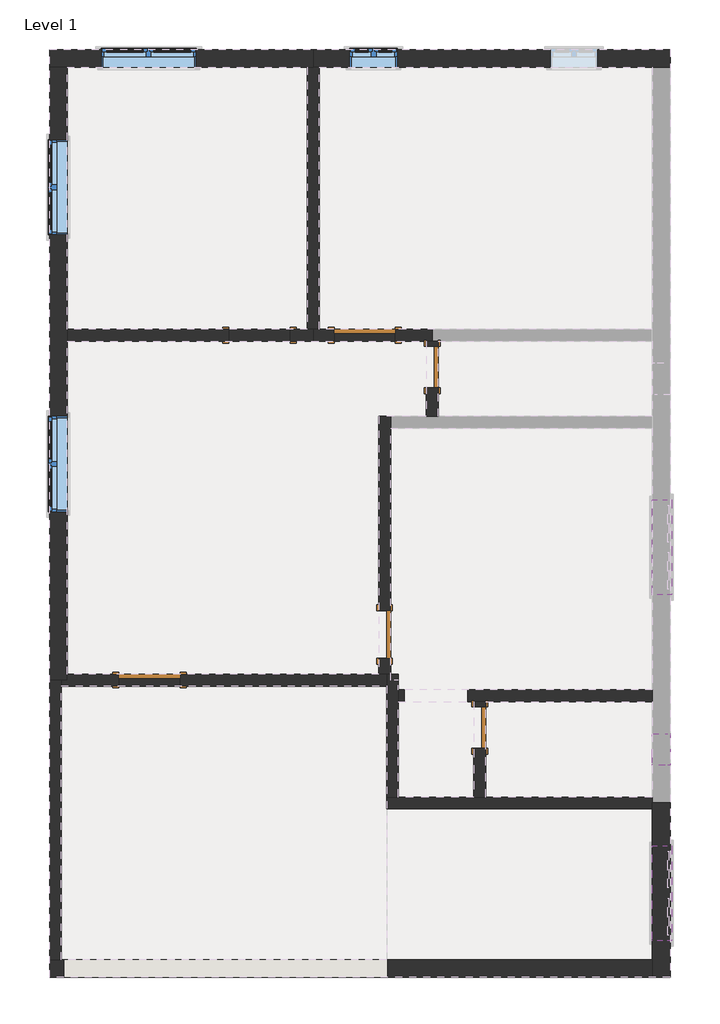
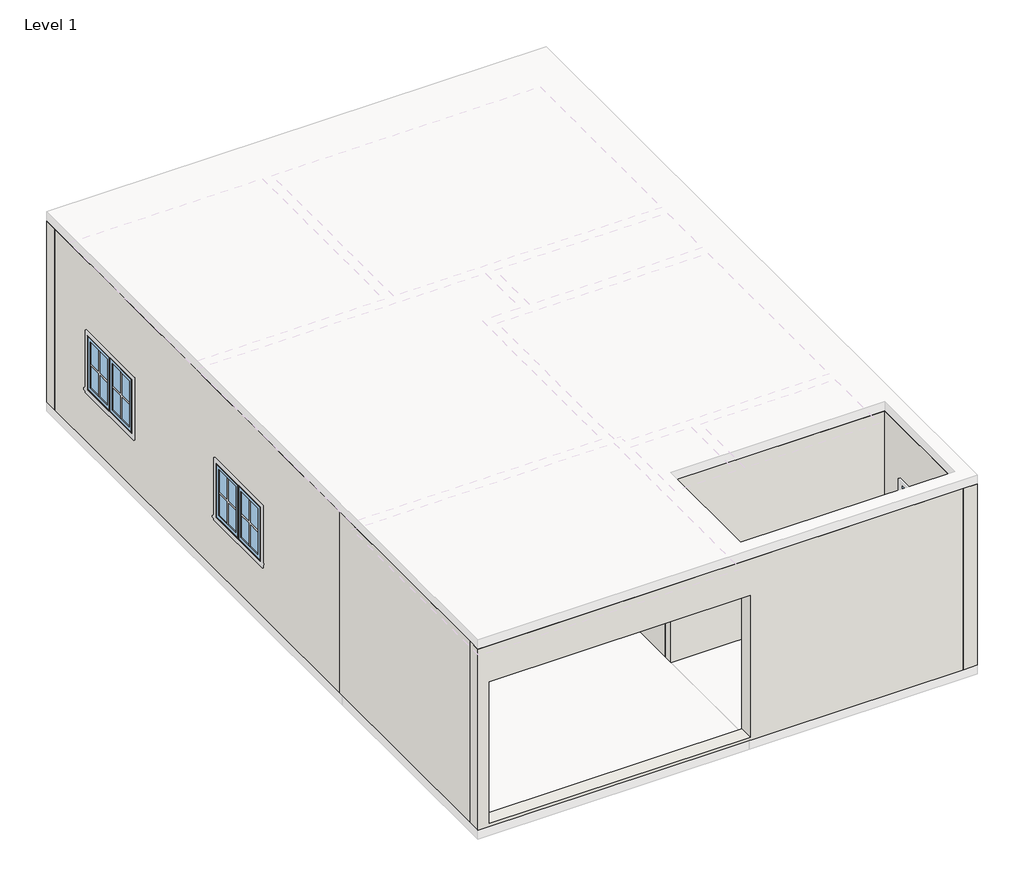
# One storey, part 1 of 2: 24 walls, 10 windows, 6 doors.
"""IFC4 building model written with IfcOpenShell, lengths in millimetres."""

from ifc_helpers import new_model, si_unit, frame, origin, origin_with_axes, place, context, project, spatial, polyline, outline, extrude, faceted_brep, transform, mapped, element, save
from components import door_2908be75, door_9ea4ff49, door_dc34e247, door_b804d09e, fixed_2_415b3208, window_casement_double_3_c417fced, window_casement_double_4_c19c33cb

model = new_model("IFC4")

# Units and contexts
model_context = context("Model", 3, world=origin())
ifc_project = project(units=[si_unit("LENGTHUNIT", "METRE", prefix="MILLI")], contexts=[model_context])

# Site, building, storey
site = spatial("IfcSite", under=ifc_project)
building = spatial("IfcBuilding", under=site)
storey = spatial("IfcBuildingStorey", under=building, Name="Level 1", Elevation=0.0)

# Doors
placement = place(None, origin())
door_shape = door_2908be75(model_context)
element("IfcDoor", 1, ObjectType="Single-Flush : 1' 9\"", at=placement, inside=storey, context=model_context, shape_type="MappedRepresentation", body=[
    mapped(door_shape, transform((-397.3154463, -2781.5544725, 0.0), x_axis=(0.0, 1.0, 0.0), y_axis=(-1.0, 0.0, 0.0), z_axis=(0.0, 0.0, 1.0))),
])
element("IfcDoor", 2, ObjectType="Single-Flush : 1' 9\"", at=placement, inside=storey, context=model_context, shape_type="MappedRepresentation", body=[
    mapped(door_shape, transform((-1006.9154463, 1841.2455275, 0.0), x_axis=(0.0, 1.0, 0.0), y_axis=(-1.0, 0.0, 0.0), z_axis=(0.0, 0.0, 1.0))),
])
door_2_shape = door_9ea4ff49(model_context)
element("IfcDoor", 3, ObjectType="Single-Flush : 2'0\"", at=placement, inside=storey, context=model_context, shape_type="MappedRepresentation", body=[
    mapped(door_2_shape, transform((-1616.5154463, -1587.7544725, 0.0), x_axis=(0.0, -1.0, 0.0), y_axis=(1.0, 0.0, 0.0), z_axis=(0.0, 0.0, 1.0))),
])
door_3_shape = door_dc34e247(model_context)
element("IfcDoor", 4, ObjectType="Single-Flush : 2'7\"", at=placement, inside=storey, context=model_context, shape_type="MappedRepresentation", body=[
    mapped(door_3_shape, transform((-4626.4154463, -2171.9544725, 0.0), x_axis=(-1.0, 0.0, 0.0), y_axis=(0.0, -1.0, 0.0), z_axis=(0.0, 0.0, 1.0))),
])
element("IfcDoor", 5, ObjectType="Single-Flush : 2'7\"", at=placement, inside=storey, context=model_context, shape_type="MappedRepresentation", body=[
    mapped(door_3_shape, transform((-1870.5154463, 2247.6455275, 0.0), x_axis=(-1.0, 0.0, 0.0), y_axis=(0.0, -1.0, 0.0), z_axis=(0.0, 0.0, 1.0))),
])
door_4_shape = door_b804d09e(model_context)
element("IfcDoor", 6, ObjectType="Single-Flush : 2'7\"", at=placement, inside=storey, context=model_context, shape_type="MappedRepresentation", body=[
    mapped(door_4_shape, transform((-3216.7154463, 2247.6455275, 0.0), x_axis=(1.0, 0.0, 0.0), y_axis=(0.0, 1.0, 0.0), z_axis=(0.0, 0.0, 1.0))),
])

# Walls
element("IfcWall", 7, ObjectType="Generic - 6\"", at=placement, inside=storey, context=model_context, shape_type="Brep", body=[
    faceted_brep([(-5909.1154463, -2171.9544725, 0.0), (-5909.1154463, -5753.3544725, 0.0), (-5909.1154463, -5753.3544725, 3048.0), (-5909.1154463, -2171.9544725, 3048.0), (-5756.7154463, -2171.9544725, 0.0), (-5756.7154463, -2171.9544725, 3048.0), (-5756.7154463, -2248.1544725, 3048.0), (-5756.7154463, -5753.3544725, 3048.0), (-5756.7154463, -5753.3544725, 0.0), (-5756.7154463, -2248.1544725, 0.0)], [[[0, 1, 2, 3]], [[4, 5, 6, 7, 8, 9]], [[1, 0, 4, 9, 8]], [[3, 2, 7, 6, 5]], [[0, 3, 5, 4]], [[2, 1, 8, 7]]]),
])
element("IfcWall", 8, ObjectType="Generic - 6\"", at=placement, inside=storey, context=model_context, shape_type="Brep", body=[
    faceted_brep([(1812.4845537, -3670.5544725, 0.0), (-321.1154463, -3670.5544725, 0.0), (-473.5154463, -3670.5544725, 0.0), (-1438.7154463, -3670.5544725, 0.0), (-1591.1154463, -3670.5544725, 0.0), (-1591.1154463, -3670.5544725, 3048.0), (-1438.7154463, -3670.5544725, 3048.0), (-473.5154463, -3670.5544725, 3048.0), (-321.1154463, -3670.5544725, 3048.0), (1812.4845537, -3670.5544725, 3048.0), (1812.4845537, -3822.9544725, 0.0), (1812.4845537, -3822.9544725, 3048.0), (-1591.1154463, -3822.9544725, 3048.0), (-1591.1154463, -3822.9544725, 0.0), (1812.4845537, -3746.7544725, 0.0), (1812.4845537, -3746.7544725, 3048.0)], [[[0, 1, 2, 3, 4, 5, 6, 7, 8, 9]], [[10, 11, 12, 13]], [[4, 3, 2, 1, 0, 14, 10, 13]], [[9, 8, 7, 6, 5, 12, 11, 15]], [[5, 4, 13, 12]], [[0, 9, 15, 11, 10, 14]]]),
])
element("IfcWall", 9, ObjectType="Generic - 6\"", at=placement, inside=storey, context=model_context, shape_type="Brep", body=[
    faceted_brep([(-1438.7154463, -3670.5544725, 0.0), (-1438.7154463, -2451.3544725, 0.0), (-1438.7154463, -2298.9544725, 0.0), (-1438.7154463, -2095.7544725, 0.0), (-1438.7154463, -2095.7544725, 3048.0), (-1438.7154463, -2298.9544725, 3048.0), (-1438.7154463, -2451.3544725, 3048.0), (-1438.7154463, -3670.5544725, 3048.0), (-1591.1154463, -3670.5544725, 0.0), (-1591.1154463, -3670.5544725, 3048.0), (-1591.1154463, -2248.1544725, 3048.0), (-1591.1154463, -2171.9544725, 3048.0), (-1591.1154463, -2095.7544725, 3048.0), (-1591.1154463, -2095.7544725, 0.0), (-1591.1154463, -2171.9544725, 0.0), (-1591.1154463, -2248.1544725, 0.0), (-1540.3154463, -2095.7544725, 0.0), (-1540.3154463, -2095.7544725, 3048.0)], [[[0, 1, 2, 3, 4, 5, 6, 7]], [[8, 9, 10, 11, 12, 13, 14, 15]], [[3, 2, 1, 0, 8, 15, 14, 13, 16]], [[7, 6, 5, 4, 17, 12, 11, 10, 9]], [[0, 7, 9, 8]], [[4, 3, 16, 13, 12, 17]]]),
])
element("IfcWall", 10, ObjectType="Generic - 6\"", at=placement, inside=storey, context=model_context, shape_type="Brep", body=[
    faceted_brep([(-5020.1154463, -2095.7544725, 2133.6), (-5020.1154463, -2095.7544725, 0.0), (-5680.5154463, -2095.7544725, 0.0), (-5680.5154463, -2095.7544725, 3048.0), (-1692.7154463, -2095.7544725, 3048.0), (-1591.1154463, -2095.7544725, 3048.0), (-1591.1154463, -2095.7544725, 0.0), (-1692.7154463, -2095.7544725, 0.0), (-4232.7154463, -2095.7544725, 0.0), (-4232.7154463, -2095.7544725, 2133.6), (-5756.7154463, -2248.1544725, 0.0), (-5020.1154463, -2248.1544725, 0.0), (-5020.1154463, -2248.1544725, 2133.6), (-4232.7154463, -2248.1544725, 2133.6), (-4232.7154463, -2248.1544725, 0.0), (-1591.1154463, -2248.1544725, 0.0), (-1591.1154463, -2248.1544725, 3048.0), (-5756.7154463, -2248.1544725, 3048.0), (-5756.7154463, -2171.9544725, 0.0), (-5680.5154463, -2171.9544725, 0.0), (-5680.5154463, -2171.9544725, 3048.0), (-5756.7154463, -2171.9544725, 3048.0)], [[[0, 1, 2, 3, 4, 5, 6, 7, 8, 9]], [[10, 11, 12, 13, 14, 15, 16, 17]], [[2, 1, 11, 10, 18, 19]], [[8, 7, 6, 15, 14]], [[5, 4, 3, 20, 21, 17, 16]], [[3, 2, 19, 20]], [[19, 18, 21, 20]], [[18, 10, 17, 21]], [[6, 5, 16, 15]], [[12, 11, 1, 0]], [[13, 12, 0, 9]], [[14, 13, 9, 8]]]),
])
element("IfcWall", 11, ObjectType="Generic - 6\"", at=placement, inside=storey, context=model_context, shape_type="Brep", body=[
    faceted_brep([(1812.4845537, -2451.3544725, 0.0), (1812.4845537, -2451.3544725, 3048.0), (-321.1154463, -2451.3544725, 3048.0), (-473.5154463, -2451.3544725, 3048.0), (-1438.7154463, -2451.3544725, 3048.0), (-1438.7154463, -2451.3544725, 0.0), (-1367.0206652, -2451.3544725, 0.0), (-1367.0206652, -2451.3544725, 2438.4), (-547.4818767, -2451.3544725, 2438.4), (-547.4818767, -2451.3544725, 0.0), (-473.5154463, -2451.3544725, 0.0), (-321.1154463, -2451.3544725, 0.0), (1812.4845537, -2298.9544725, 3048.0), (1812.4845537, -2298.9544725, 0.0), (-547.4818767, -2298.9544725, 0.0), (-547.4818767, -2298.9544725, 2438.4), (-1367.0206652, -2298.9544725, 2438.4), (-1367.0206652, -2298.9544725, 0.0), (-1438.7154463, -2298.9544725, 0.0), (-1438.7154463, -2298.9544725, 3048.0)], [[[0, 1, 2, 3, 4, 5, 6, 7, 8, 9, 10, 11]], [[12, 13, 14, 15, 16, 17, 18, 19]], [[5, 18, 17, 6]], [[13, 0, 11, 10, 9, 14]], [[4, 3, 2, 1, 12, 19]], [[1, 0, 13, 12]], [[5, 4, 19, 18]], [[7, 16, 15, 8]], [[16, 7, 6, 17]], [[8, 15, 14, 9]]]),
])
element("IfcWall", 12, ObjectType="Generic - 6\"", at=placement, inside=storey, context=model_context, shape_type="SweptSolid", body=[
    extrude(outline(polyline([(-2451.3544725, 0.0), (-2514.8544725, 0.0), (-2514.8544725, 2133.6), (-3048.2544725, 2133.6), (-3048.2544725, 0.0), (-3670.5544725, 0.0), (-3670.5544725, 3048.0), (-2451.3544725, 3048.0), (-2451.3544725, 0.0)])), frame((-473.5154463, 0.0, 0.0), z_axis=(1.0, 0.0, 0.0), x_axis=(0.0, 1.0, 0.0)), (0.0, 0.0, 1.0), 152.4),
])
element("IfcWall", 13, ObjectType="Generic - 6\"", at=placement, inside=storey, context=model_context, shape_type="Brep", body=[
    faceted_brep([(-1540.3154463, -2095.7544725, 0.0), (-1540.3154463, -1892.5544725, 0.0), (-1540.3154463, -1892.5544725, 2133.6), (-1540.3154463, -1282.9544725, 2133.6), (-1540.3154463, -1282.9544725, 0.0), (-1540.3154463, 1053.8455275, 0.0), (-1540.3154463, 1206.2455275, 0.0), (-1540.3154463, 1206.2455275, 3048.0), (-1540.3154463, 1053.8455275, 3048.0), (-1540.3154463, -2095.7544725, 3048.0), (-1692.7154463, -1892.5544725, 2133.6), (-1692.7154463, -1892.5544725, 0.0), (-1692.7154463, -2095.7544725, 0.0), (-1692.7154463, -2095.7544725, 3048.0), (-1692.7154463, 1206.2455275, 3048.0), (-1692.7154463, 1206.2455275, 0.0), (-1692.7154463, -1282.9544725, 0.0), (-1692.7154463, -1282.9544725, 2133.6), (-1591.1154463, -2095.7544725, 0.0), (-1591.1154463, -2095.7544725, 3048.0)], [[[0, 1, 2, 3, 4, 5, 6, 7, 8, 9]], [[10, 11, 12, 13, 14, 15, 16, 17]], [[16, 15, 6, 5, 4]], [[12, 11, 1, 0, 18]], [[9, 8, 7, 14, 13, 19]], [[0, 9, 19, 13, 12, 18]], [[7, 6, 15, 14]], [[2, 1, 11, 10]], [[3, 2, 10, 17]], [[4, 3, 17, 16]]]),
])
element("IfcWall", 14, ObjectType="Generic - 6\"", at=placement, inside=storey, context=model_context, shape_type="Brep", body=[
    faceted_brep([(-930.7154463, 2107.9455275, 2133.6), (-930.7154463, 2107.9455275, 0.0), (-930.7154463, 2171.4455275, 0.0), (-930.7154463, 2171.4455275, 3048.0), (-930.7154463, 1206.2455275, 3048.0), (-930.7154463, 1206.2455275, 0.0), (-930.7154463, 1574.5455275, 0.0), (-930.7154463, 1574.5455275, 2133.6), (-1083.1154463, 2171.4455275, 0.0), (-1083.1154463, 2107.9455275, 0.0), (-1083.1154463, 2107.9455275, 2133.6), (-1083.1154463, 1574.5455275, 2133.6), (-1083.1154463, 1574.5455275, 0.0), (-1083.1154463, 1206.2455275, 0.0), (-1083.1154463, 1206.2455275, 3048.0), (-1083.1154463, 2171.4455275, 3048.0), (-1006.9154463, 2171.4455275, 0.0), (-1006.9154463, 2171.4455275, 3048.0)], [[[0, 1, 2, 3, 4, 5, 6, 7]], [[8, 9, 10, 11, 12, 13, 14, 15]], [[6, 5, 13, 12]], [[2, 1, 9, 8, 16]], [[4, 3, 17, 15, 14]], [[5, 4, 14, 13]], [[10, 9, 1, 0]], [[11, 10, 0, 7]], [[12, 11, 7, 6]], [[3, 2, 16, 8, 15, 17]]]),
])
element("IfcWall", 15, ObjectType="Generic - 6\"", at=placement, inside=storey, context=model_context, shape_type="Brep", body=[
    faceted_brep([(-2607.1154463, 5678.2330275, 0.0), (-2607.1154463, 2323.8455275, 0.0), (-2607.1154463, 2323.8455275, 3048.0), (-2607.1154463, 5678.2330275, 3048.0), (-2454.7154463, 5678.2330275, 0.0), (-2454.7154463, 5678.2330275, 3048.0), (-2454.7154463, 2323.8455275, 3048.0), (-2454.7154463, 2323.8455275, 0.0), (-2530.9154463, 5678.2330275, 0.0), (-2530.9154463, 2323.8455275, 0.0), (-2530.9154463, 2323.8455275, 3048.0), (-2530.9154463, 5678.2330275, 3048.0)], [[[0, 1, 2, 3]], [[4, 5, 6, 7]], [[1, 0, 8, 4, 7, 9]], [[3, 2, 10, 6, 5, 11]], [[0, 3, 11, 5, 4, 8]], [[2, 1, 9, 7, 6, 10]]]),
])
element("IfcWall", 16, ObjectType="Generic - 6\"", at=placement, inside=storey, context=model_context, shape_type="Brep", body=[
    faceted_brep([(-2530.9154463, 2323.8455275, 0.0), (-2607.1154463, 2323.8455275, 0.0), (-2823.0154463, 2323.8455275, 0.0), (-2823.0154463, 2323.8455275, 2133.6), (-3610.4154463, 2323.8455275, 2133.6), (-3610.4154463, 2323.8455275, 0.0), (-5680.5154463, 2323.8455275, 0.0), (-5680.5154463, 2323.8455275, 3048.0), (-2607.1154463, 2323.8455275, 3048.0), (-2530.9154463, 2323.8455275, 3048.0), (-2823.0154463, 2171.4455275, 2133.6), (-2823.0154463, 2171.4455275, 0.0), (-2530.9154463, 2171.4455275, 0.0), (-2530.9154463, 2171.4455275, 3048.0), (-5680.5154463, 2171.4455275, 3048.0), (-5680.5154463, 2171.4455275, 0.0), (-3610.4154463, 2171.4455275, 0.0), (-3610.4154463, 2171.4455275, 2133.6)], [[[0, 1, 2, 3, 4, 5, 6, 7, 8, 9]], [[10, 11, 12, 13, 14, 15, 16, 17]], [[16, 15, 6, 5]], [[12, 11, 2, 1, 0]], [[9, 8, 7, 14, 13]], [[0, 9, 13, 12]], [[7, 6, 15, 14]], [[5, 4, 17, 16]], [[4, 3, 10, 17]], [[3, 2, 11, 10]]]),
])
element("IfcWall", 17, ObjectType="Generic - 6\"", at=placement, inside=storey, context=model_context, shape_type="Brep", body=[
    faceted_brep([(-2264.2154463, 2323.8455275, 2133.6), (-2264.2154463, 2323.8455275, 0.0), (-2454.7154463, 2323.8455275, 0.0), (-2530.9154463, 2323.8455275, 0.0), (-2530.9154463, 2323.8455275, 3048.0), (-2454.7154463, 2323.8455275, 3048.0), (-1006.9154463, 2323.8455275, 3048.0), (-1006.9154463, 2323.8455275, 0.0), (-1476.8154463, 2323.8455275, 0.0), (-1476.8154463, 2323.8455275, 2133.6), (-2530.9154463, 2171.4455275, 0.0), (-2264.2154463, 2171.4455275, 0.0), (-2264.2154463, 2171.4455275, 2133.6), (-1476.8154463, 2171.4455275, 2133.6), (-1476.8154463, 2171.4455275, 0.0), (-1083.1154463, 2171.4455275, 0.0), (-1006.9154463, 2171.4455275, 0.0), (-1006.9154463, 2171.4455275, 3048.0), (-1083.1154463, 2171.4455275, 3048.0), (-2530.9154463, 2171.4455275, 3048.0)], [[[0, 1, 2, 3, 4, 5, 6, 7, 8, 9]], [[10, 11, 12, 13, 14, 15, 16, 17, 18, 19]], [[8, 7, 16, 15, 14]], [[3, 2, 1, 11, 10]], [[4, 3, 10, 19]], [[6, 5, 4, 19, 18, 17]], [[7, 6, 17, 16]], [[14, 13, 9, 8]], [[13, 12, 0, 9]], [[12, 11, 1, 0]]]),
])
element("IfcWall", 18, ObjectType="Generic - 6\"", at=placement, inside=storey, context=model_context, shape_type="SweptSolid", body=[
    extrude(outline(polyline([(-5680.5154463, -2095.7544725), (-1692.7154463, -2095.7544725), (-1692.7154463, -2171.9544725), (-1591.1154463, -2171.9544725), (-1591.1154463, -2248.1544725), (-5756.7154463, -2248.1544725), (-5756.7154463, -2171.9544725), (-5680.5154463, -2171.9544725), (-5680.5154463, -2095.7544725)])), origin_with_axes(), (0.0, 0.0, 1.0), 3048.0),
])
element("IfcWall", 19, ObjectType="Generic - 6\"", at=placement, inside=storey, context=model_context, shape_type="Brep", body=[
    faceted_brep([(-2607.1154463, 5678.2330275, 0.0), (-2607.1154463, 2323.8455275, 0.0), (-2607.1154463, 2323.8455275, 3048.0), (-2607.1154463, 5678.2330275, 3048.0), (-2454.7154463, 5678.2330275, 0.0), (-2454.7154463, 5678.2330275, 3048.0), (-2454.7154463, 2323.8455275, 3048.0), (-2454.7154463, 2323.8455275, 0.0), (-2530.9154463, 5678.2330275, 0.0), (-2530.9154463, 2323.8455275, 0.0), (-2530.9154463, 2323.8455275, 3048.0), (-2530.9154463, 5678.2330275, 3048.0)], [[[0, 1, 2, 3]], [[4, 5, 6, 7]], [[1, 0, 8, 4, 7, 9]], [[3, 2, 10, 6, 5, 11]], [[0, 3, 11, 5, 4, 8]], [[2, 1, 9, 7, 6, 10]]]),
])
element("IfcWall", 20, ObjectType="Generic - 6\"", at=placement, inside=storey, context=model_context, shape_type="Brep", body=[
    faceted_brep([(-2530.9154463, 2323.8455275, 0.0), (-2607.1154463, 2323.8455275, 0.0), (-5680.5154463, 2323.8455275, 0.0), (-5680.5154463, 2323.8455275, 3048.0), (-2607.1154463, 2323.8455275, 3048.0), (-2530.9154463, 2323.8455275, 3048.0), (-2530.9154463, 2171.4455275, 0.0), (-2530.9154463, 2171.4455275, 3048.0), (-5680.5154463, 2171.4455275, 3048.0), (-5680.5154463, 2171.4455275, 0.0)], [[[0, 1, 2, 3, 4, 5]], [[6, 7, 8, 9]], [[2, 1, 0, 6, 9]], [[5, 4, 3, 8, 7]], [[0, 5, 7, 6]], [[3, 2, 9, 8]]]),
])
element("IfcWall", 21, ObjectType="Generic - 6\"", at=placement, inside=storey, context=model_context, shape_type="Brep", body=[
    faceted_brep([(-1006.9154463, 2323.8455275, 0.0), (-2454.7154463, 2323.8455275, 0.0), (-2530.9154463, 2323.8455275, 0.0), (-2530.9154463, 2323.8455275, 3048.0), (-2454.7154463, 2323.8455275, 3048.0), (-1006.9154463, 2323.8455275, 3048.0), (-1006.9154463, 2171.4455275, 0.0), (-1006.9154463, 2171.4455275, 3048.0), (-1083.1154463, 2171.4455275, 3048.0), (-2530.9154463, 2171.4455275, 3048.0), (-2530.9154463, 2171.4455275, 0.0), (-1083.1154463, 2171.4455275, 0.0)], [[[0, 1, 2, 3, 4, 5]], [[6, 7, 8, 9, 10, 11]], [[2, 1, 0, 6, 11, 10]], [[3, 2, 10, 9]], [[5, 4, 3, 9, 8, 7]], [[0, 5, 7, 6]]]),
])
element("IfcWall", 22, ObjectType="Generic - 9\"", at=placement, inside=storey, context=model_context, shape_type="Brep", body=[
    faceted_brep([(-5909.1154463, 5678.2330275, 0.0), (-5680.5154463, 5678.2330275, 0.0), (-2607.1154463, 5678.2330275, 0.0), (-2530.9154463, 5678.2330275, 0.0), (-2530.9154463, 5678.2330275, 3048.0), (-2607.1154463, 5678.2330275, 3048.0), (-5680.5154463, 5678.2330275, 3048.0), (-5909.1154463, 5678.2330275, 3048.0), (-4029.5154463, 5678.2330275, 1828.8), (-4029.5154463, 5678.2330275, 914.4), (-5248.7154463, 5678.2330275, 914.4), (-5248.7154463, 5678.2330275, 1828.8), (-5909.1154463, 5906.8330275, 0.0), (-5909.1154463, 5906.8330275, 3048.0), (-2530.9154463, 5906.8330275, 3048.0), (-2530.9154463, 5906.8330275, 0.0), (-4029.5154463, 5906.8330275, 1828.8), (-5248.7154463, 5906.8330275, 1828.8), (-5248.7154463, 5906.8330275, 914.4), (-4029.5154463, 5906.8330275, 914.4)], [[[0, 1, 2, 3, 4, 5, 6, 7], [8, 9, 10, 11]], [[12, 13, 14, 15], [16, 17, 18, 19]], [[3, 2, 1, 0, 12, 15]], [[4, 3, 15, 14]], [[7, 6, 5, 4, 14, 13]], [[0, 7, 13, 12]], [[9, 8, 16, 19]], [[10, 9, 19, 18]], [[11, 10, 18, 17]], [[8, 11, 17, 16]]]),
])
element("IfcWall", 23, ObjectType="Generic - 9\"", at=placement, inside=storey, context=model_context, shape_type="Brep", body=[
    faceted_brep([(1812.4845537, -5753.3544725, 0.0), (-5756.7154463, -5753.3544725, 0.0), (-5909.1154463, -5753.3544725, 0.0), (-5909.1154463, -5753.3544725, 3048.0), (-5756.7154463, -5753.3544725, 3048.0), (1812.4845537, -5753.3544725, 3048.0), (-1576.8982041, -5753.3544725, 2438.4), (-5729.1673724, -5753.3544725, 2438.4), (-5729.1673724, -5753.3544725, 50.8), (-1576.8982041, -5753.3544725, 50.8), (-5909.1154463, -5981.9544725, 0.0), (1812.4845537, -5981.9544725, 0.0), (1812.4845537, -5981.9544725, 3048.0), (-5909.1154463, -5981.9544725, 3048.0), (-5729.1673724, -5981.9544725, 2438.4), (-1576.8982041, -5981.9544725, 2438.4), (-1576.8982041, -5981.9544725, 50.8), (-5729.1673724, -5981.9544725, 50.8)], [[[0, 1, 2, 3, 4, 5], [6, 7, 8, 9]], [[10, 11, 12, 13], [14, 15, 16, 17]], [[2, 1, 0, 11, 10]], [[5, 4, 3, 13, 12]], [[0, 5, 12, 11]], [[6, 15, 14, 7]], [[8, 17, 16, 9]], [[15, 6, 9, 16]], [[7, 14, 17, 8]], [[3, 2, 10, 13]]]),
])
element("IfcWall", 24, ObjectType="Generic - 9\"", at=placement, inside=storey, context=model_context, shape_type="Brep", body=[
    faceted_brep([(-5909.1154463, 5678.2330275, 0.0), (-5909.1154463, -2171.9544725, 0.0), (-5909.1154463, -2171.9544725, 3048.0), (-5909.1154463, 5678.2330275, 3048.0), (-5909.1154463, 4751.1330275, 1828.8), (-5909.1154463, 3531.9330275, 1828.8), (-5909.1154463, 3531.9330275, 914.4), (-5909.1154463, 4751.1330275, 914.4), (-5909.1154463, 1206.2455275, 1828.8), (-5909.1154463, -12.9544725, 1828.8), (-5909.1154463, -12.9544725, 914.4), (-5909.1154463, 1206.2455275, 914.4), (-5680.5154463, 5678.2330275, 0.0), (-5680.5154463, 5678.2330275, 3048.0), (-5680.5154463, 2323.8455275, 3048.0), (-5680.5154463, 2171.4455275, 3048.0), (-5680.5154463, -2095.7544725, 3048.0), (-5680.5154463, -2171.9544725, 3048.0), (-5680.5154463, -2171.9544725, 0.0), (-5680.5154463, -2095.7544725, 0.0), (-5680.5154463, 2171.4455275, 0.0), (-5680.5154463, 2323.8455275, 0.0), (-5680.5154463, 4751.1330275, 1828.8), (-5680.5154463, 4751.1330275, 914.4), (-5680.5154463, 3531.9330275, 914.4), (-5680.5154463, 3531.9330275, 1828.8), (-5680.5154463, 1206.2455275, 1828.8), (-5680.5154463, 1206.2455275, 914.4), (-5680.5154463, -12.9544725, 914.4), (-5680.5154463, -12.9544725, 1828.8), (-5756.7154463, -2171.9544725, 0.0), (-5756.7154463, -2171.9544725, 3048.0)], [[[0, 1, 2, 3], [4, 5, 6, 7], [8, 9, 10, 11]], [[12, 13, 14, 15, 16, 17, 18, 19, 20, 21], [22, 23, 24, 25], [26, 27, 28, 29]], [[1, 0, 12, 21, 20, 19, 18, 30]], [[2, 1, 30, 18, 17, 31]], [[3, 2, 31, 17, 16, 15, 14, 13]], [[0, 3, 13, 12]], [[23, 22, 4, 7]], [[24, 23, 7, 6]], [[25, 24, 6, 5]], [[22, 25, 5, 4]], [[27, 26, 8, 11]], [[28, 27, 11, 10]], [[29, 28, 10, 9]], [[26, 29, 9, 8]]]),
])
element("IfcWall", 25, ObjectType="Generic - 9\"", at=placement, inside=storey, context=model_context, shape_type="Brep", body=[
    faceted_brep([(-2530.9154463, 5678.2330275, 0.0), (-2454.7154463, 5678.2330275, 0.0), (1812.4845537, 5678.2330275, 0.0), (2041.0845537, 5678.2330275, 0.0), (2041.0845537, 5678.2330275, 3048.0), (1812.4845537, 5678.2330275, 3048.0), (-2454.7154463, 5678.2330275, 3048.0), (-2530.9154463, 5678.2330275, 3048.0), (-1451.4154463, 5678.2330275, 1828.8), (-1451.4154463, 5678.2330275, 914.4), (-2061.0154463, 5678.2330275, 914.4), (-2061.0154463, 5678.2330275, 1828.8), (1113.9845537, 5678.2330275, 1828.8), (1113.9845537, 5678.2330275, 914.4), (504.3845537, 5678.2330275, 914.4), (504.3845537, 5678.2330275, 1828.8), (-2530.9154463, 5906.8330275, 0.0), (-2530.9154463, 5906.8330275, 3048.0), (2041.0845537, 5906.8330275, 3048.0), (2041.0845537, 5906.8330275, 0.0), (-1451.4154463, 5906.8330275, 1828.8), (-2061.0154463, 5906.8330275, 1828.8), (-2061.0154463, 5906.8330275, 914.4), (-1451.4154463, 5906.8330275, 914.4), (1113.9845537, 5906.8330275, 1828.8), (504.3845537, 5906.8330275, 1828.8), (504.3845537, 5906.8330275, 914.4), (1113.9845537, 5906.8330275, 914.4)], [[[0, 1, 2, 3, 4, 5, 6, 7], [8, 9, 10, 11], [12, 13, 14, 15]], [[16, 17, 18, 19], [20, 21, 22, 23], [24, 25, 26, 27]], [[3, 2, 1, 0, 16, 19]], [[7, 6, 5, 4, 18, 17]], [[0, 7, 17, 16]], [[4, 3, 19, 18]], [[8, 11, 21, 20]], [[11, 10, 22, 21]], [[10, 9, 23, 22]], [[9, 8, 20, 23]], [[12, 15, 25, 24]], [[15, 14, 26, 25]], [[14, 13, 27, 26]], [[13, 12, 24, 27]]]),
])
element("IfcWall", 26, ObjectType="Generic - 9\"", at=placement, inside=storey, context=model_context, shape_type="Brep", body=[
    faceted_brep([(1812.4845537, -3746.7544725, 0.0), (1812.4845537, -3822.9544725, 0.0), (1812.4845537, -5753.3544725, 0.0), (1812.4845537, -5981.9544725, 0.0), (1812.4845537, -5981.9544725, 3048.0), (1812.4845537, -5753.3544725, 3048.0), (1812.4845537, -3822.9544725, 3048.0), (1812.4845537, -3746.7544725, 3048.0), (1812.4845537, -5512.0544725, 2133.6), (1812.4845537, -5512.0544725, 1219.2), (1812.4845537, -4292.8544725, 1219.2), (1812.4845537, -4292.8544725, 2133.6), (2041.0845537, -3746.7544725, 0.0), (2041.0845537, -3746.7544725, 3048.0), (2041.0845537, -5981.9544725, 3048.0), (2041.0845537, -5981.9544725, 0.0), (2041.0845537, -5512.0544725, 2133.6), (2041.0845537, -4292.8544725, 2133.6), (2041.0845537, -4292.8544725, 1219.2), (2041.0845537, -5512.0544725, 1219.2)], [[[0, 1, 2, 3, 4, 5, 6, 7], [8, 9, 10, 11]], [[12, 13, 14, 15], [16, 17, 18, 19]], [[3, 2, 1, 0, 12, 15]], [[7, 6, 5, 4, 14, 13]], [[0, 7, 13, 12]], [[4, 3, 15, 14]], [[8, 11, 17, 16]], [[11, 10, 18, 17]], [[10, 9, 19, 18]], [[9, 8, 16, 19]]]),
])
element("IfcWall", 27, ObjectType="Generic - 9\"", at=placement, inside=storey, context=model_context, shape_type="SweptSolid", body=[
    extrude(outline(polyline([(0.0, -5680.5154463), (0.0, -2607.1154463), (3048.0, -2607.1154463), (3048.0, -5680.5154463), (0.0, -5680.5154463)]), holes=[polyline([(1828.8, -4029.5154463), (914.4, -4029.5154463), (914.4, -5248.7154463), (1828.8, -5248.7154463), (1828.8, -4029.5154463)])]), frame((0.0, 5678.2330275, 0.0), z_axis=(0.0, 1.0, 0.0), x_axis=(0.0, 0.0, 1.0)), (0.0, 0.0, 1.0), 228.6),
])
element("IfcWall", 28, ObjectType="Generic - 9\"", at=placement, inside=storey, context=model_context, shape_type="Brep", body=[
    faceted_brep([(1812.4845537, -5753.3544725, 0.0), (-5756.7154463, -5753.3544725, 0.0), (-5909.1154463, -5753.3544725, 0.0), (-5909.1154463, -5753.3544725, 3048.0), (-5756.7154463, -5753.3544725, 3048.0), (1812.4845537, -5753.3544725, 3048.0), (-1576.8982041, -5753.3544725, 2438.4), (-5729.1673724, -5753.3544725, 2438.4), (-5729.1673724, -5753.3544725, 50.8), (-1576.8982041, -5753.3544725, 50.8), (-5909.1154463, -5981.9544725, 0.0), (1812.4845537, -5981.9544725, 0.0), (1812.4845537, -5981.9544725, 3048.0), (-5909.1154463, -5981.9544725, 3048.0), (-5729.1673724, -5981.9544725, 2438.4), (-1576.8982041, -5981.9544725, 2438.4), (-1576.8982041, -5981.9544725, 50.8), (-5729.1673724, -5981.9544725, 50.8)], [[[0, 1, 2, 3, 4, 5], [6, 7, 8, 9]], [[10, 11, 12, 13], [14, 15, 16, 17]], [[2, 1, 0, 11, 10]], [[5, 4, 3, 13, 12]], [[6, 15, 14, 7]], [[8, 17, 16, 9]], [[15, 6, 9, 16]], [[7, 14, 17, 8]], [[3, 2, 10, 13]], [[0, 5, 12, 11]]]),
])
element("IfcWall", 29, ObjectType="Generic - 9\"", at=placement, inside=storey, context=model_context, shape_type="SweptSolid", body=[
    extrude(outline(polyline([(0.0, -2454.7154463), (0.0, 1812.4845537), (3048.0, 1812.4845537), (3048.0, -2454.7154463), (0.0, -2454.7154463)]), holes=[polyline([(1828.8, -1451.4154463), (914.4, -1451.4154463), (914.4, -2061.0154463), (1828.8, -2061.0154463), (1828.8, -1451.4154463)]), polyline([(1828.8, 1113.9845537), (914.4, 1113.9845537), (914.4, 504.3845537), (1828.8, 504.3845537), (1828.8, 1113.9845537)])]), frame((0.0, 5678.2330275, 0.0), z_axis=(0.0, 1.0, 0.0), x_axis=(0.0, 0.0, 1.0)), (0.0, 0.0, 1.0), 228.6),
])
element("IfcWall", 30, ObjectType="Generic - 9\"", at=placement, inside=storey, context=model_context, shape_type="SweptSolid", body=[
    extrude(outline(polyline([(-3822.9544725, 0.0), (-5753.3544725, 0.0), (-5753.3544725, 3048.0), (-3822.9544725, 3048.0), (-3822.9544725, 0.0)]), holes=[polyline([(-5512.0544725, 2133.6), (-5512.0544725, 1219.2), (-4292.8544725, 1219.2), (-4292.8544725, 2133.6), (-5512.0544725, 2133.6)])]), frame((1812.4845537, 0.0, 0.0), z_axis=(1.0, 0.0, 0.0), x_axis=(0.0, 1.0, 0.0)), (0.0, 0.0, 1.0), 228.6),
])

# Windows
fixed_2_shape = fixed_2_415b3208(model_context)
element("IfcWindow", 31, ObjectType="Fixed : 2'", at=placement, inside=storey, context=model_context, shape_type="MappedRepresentation", body=[
    mapped(fixed_2_shape, transform((1926.7845537, -3099.0544725, 1524.0), x_axis=(0.0, -1.0, 0.0), y_axis=(1.0, 0.0, 0.0), z_axis=(0.0, 0.0, 1.0))),
])
window_casement_double_3_shape = window_casement_double_3_c417fced(model_context)
element("IfcWindow", 32, ObjectType="Window-Casement-Double : 3'", at=placement, inside=storey, context=model_context, shape_type="MappedRepresentation", body=[
    mapped(window_casement_double_3_shape, transform((-1756.2154463, 5792.5330275, 0.0), x_axis=(1.0, 0.0, 0.0), y_axis=(0.0, 1.0, 0.0), z_axis=(0.0, 0.0, 1.0))),
])
element("IfcWindow", 33, ObjectType="Window-Casement-Double : 3'", at=placement, inside=storey, context=model_context, shape_type="MappedRepresentation", body=[
    mapped(window_casement_double_3_shape, transform((-1756.2154463, 5792.5330275, 0.0), x_axis=(1.0, 0.0, 0.0), y_axis=(0.0, 1.0, 0.0), z_axis=(0.0, 0.0, 1.0))),
])
window_casement_double_4_shape = window_casement_double_4_c19c33cb(model_context)
element("IfcWindow", 34, ObjectType="Window-Casement-Double : 4'", at=placement, inside=storey, context=model_context, shape_type="MappedRepresentation", body=[
    mapped(window_casement_double_4_shape, transform((-4639.1154463, 5792.5330275, 0.0), x_axis=(1.0, 0.0, 0.0), y_axis=(0.0, 1.0, 0.0), z_axis=(0.0, 0.0, 1.0))),
])
element("IfcWindow", 35, ObjectType="Window-Casement-Double : 4'", at=placement, inside=storey, context=model_context, shape_type="MappedRepresentation", body=[
    mapped(window_casement_double_4_shape, transform((-5794.8154463, 4141.5330275, 0.0), x_axis=(0.0, 1.0, 0.0), y_axis=(-1.0, 0.0, 0.0), z_axis=(0.0, 0.0, 1.0))),
])
element("IfcWindow", 36, ObjectType="Window-Casement-Double : 4'", at=placement, inside=storey, context=model_context, shape_type="MappedRepresentation", body=[
    mapped(window_casement_double_4_shape, transform((-5794.8154463, 596.6455275, 0.0), x_axis=(0.0, 1.0, 0.0), y_axis=(-1.0, 0.0, 0.0), z_axis=(0.0, 0.0, 1.0))),
])
element("IfcWindow", 37, ObjectType="Window-Casement-Double : 4'", at=placement, inside=storey, context=model_context, shape_type="MappedRepresentation", body=[
    mapped(window_casement_double_4_shape, transform((1926.7845537, -470.1544725, 304.8), x_axis=(0.0, -1.0, 0.0), y_axis=(1.0, 0.0, 0.0), z_axis=(0.0, 0.0, 1.0))),
])
element("IfcWindow", 38, ObjectType="Window-Casement-Double : 4'", at=placement, inside=storey, context=model_context, shape_type="MappedRepresentation", body=[
    mapped(window_casement_double_4_shape, transform((1926.7845537, -4902.4544725, 304.8), x_axis=(0.0, -1.0, 0.0), y_axis=(1.0, 0.0, 0.0), z_axis=(0.0, 0.0, 1.0))),
])
element("IfcWindow", 39, ObjectType="Window-Casement-Double : 4'", at=placement, inside=storey, context=model_context, shape_type="MappedRepresentation", body=[
    mapped(window_casement_double_4_shape, transform((-4639.1154463, 5792.5330275, 0.0), x_axis=(1.0, 0.0, 0.0), y_axis=(0.0, 1.0, 0.0), z_axis=(0.0, 0.0, 1.0))),
])
element("IfcWindow", 40, ObjectType="Window-Casement-Double : 4'", at=placement, inside=storey, context=model_context, shape_type="MappedRepresentation", body=[
    mapped(window_casement_double_4_shape, transform((1926.7845537, -4902.4544725, 304.8), x_axis=(0.0, -1.0, 0.0), y_axis=(1.0, 0.0, 0.0), z_axis=(0.0, 0.0, 1.0))),
])

save(model, "model.ifc")

# Revit data of these elements
# Type "Single-Flush : 1' 9\""
#   Type Mark = "10"
#   Construction Type Id = "MDOOR"
#   Assembly Code = "C1020"
#   Analytic Construction = "Metal"
#   Thickness = 0' - 2"
#   Heat Transfer Coefficient (U) = 0.651978 BTU/(h·ft²·°F)
#   Height = 7' - 0"
#   Trim Projection Ext = 0' - 1"
#   Trim Projection Int = 0' - 1"
#   Trim Width = 0' - 3"
#   Width = 1' - 9"
#   Define Thermal Properties by = 1
#   Door Material = Door - Panel
#   Frame Material = Door - Frame
#   Visual Light Transmittance = 0
#   Solar Heat Gain Coefficient = 0
#   Function = (empty or 0)
#   Wall Closure = (empty or 0)
# Type "Single-Flush : 2'0\""
#   Type Mark = "9"
#   Construction Type Id = "MDOOR"
#   Assembly Code = "C1020"
#   Analytic Construction = "Metal"
#   Thickness = 0' - 2"
#   Heat Transfer Coefficient (U) = 0.651978 BTU/(h·ft²·°F)
#   Height = 7' - 0"
#   Trim Projection Ext = 0' - 1"
#   Trim Projection Int = 0' - 1"
#   Trim Width = 0' - 3"
#   Width = 2' - 0"
#   Define Thermal Properties by = 1
#   Door Material = Door - Panel
#   Frame Material = Door - Frame
#   Visual Light Transmittance = 0
#   Solar Heat Gain Coefficient = 0
#   Function = (empty or 0)
#   Wall Closure = (empty or 0)
# Type "Single-Flush : 2'7\""
#   Type Mark = "8"
#   Construction Type Id = "MDOOR"
#   Assembly Code = "C1020"
#   Analytic Construction = "Metal"
#   Thickness = 0' - 2"
#   Heat Transfer Coefficient (U) = 0.651978 BTU/(h·ft²·°F)
#   Height = 7' - 0"
#   Trim Projection Ext = 0' - 1"
#   Trim Projection Int = 0' - 1"
#   Trim Width = 0' - 3"
#   Width = 2' - 7"
#   Define Thermal Properties by = 1
#   Door Material = Door - Panel
#   Frame Material = Door - Frame
#   Visual Light Transmittance = 0
#   Solar Heat Gain Coefficient = 0
#   Function = (empty or 0)
#   Wall Closure = (empty or 0)
# Type "Generic - 6\""
#   Assembly Code = "B2010"
#   Layers, outside or top first: 0' - 6" no material (function 1)
# Type "Generic - 9\""
#   Assembly Code = "B2010"
#   Layers, outside or top first: 0' - 9" no material (function 1)
# Type "Fixed : 2'"
#   Type Mark = "20"
#   Construction Type Id = "GSP4R"
#   Assembly Code = "B2020100"
#   Analytic Construction = "1/8 in Pilkington single glazing"
#   Visual Light Transmittance = 0.9
#   Solar Heat Gain Coefficient = 0.78
#   Heat Transfer Coefficient (U) = 0.6496 BTU/(h·ft²·°F)
#   Height = 2' - 0"
#   Default Sill Height = 1' - 0"
#   Width = 1' - 4"
#   Window Inset = 0' - 0 3/4"
#   Define Thermal Properties by = 1
#   Glass Pane Material = Glass
#   Sash Material = Sash
#   Wall Closure = (empty or 0)
# Type "Window-Casement-Double : 3'"
#   Type Mark = "19"
#   Fire Rating = "0.5h"
#   Assembly Code = "B2020100"
#   Analytic Construction = "Double glazing - domestic"
#   Frame Extension [instance default] = 0' - 0 1/4"
#   Window Inset [instance default] = 0' - 0"
#   Wall Thickness [instance default] = 0' - 6"
#   Interior Wall Closure [instance default] = 0' - 2 1/4"
#   Half Width = 1' - 0"
#   Visual Light Transmittance = 0.81
#   Thermal Resistance (R) = 1.8146 (h·ft²·°F)/BTU
#   Solar Heat Gain Coefficient = 0.76
#   Rough Width = 2' - 0 1/2"
#   Rough Height = 3' - 0 1/2"
#   Height = 3' - 0"
#   Heat Transfer Coefficient (U) = 0.5511 BTU/(h·ft²·°F)
#   Exterior Wall Closure [instance default] = 0' - 1 1/4"
#   Extension Jamb [instance default] = 0' - 2 1/4"
#   Default Sill Height = 3' - 0"
#   Width = 2' - 0"
#   Muntin Visibility = yes
#   Interior Trim Visibility [instance default] = yes
#   Exterior Trim Visibility [instance default] = yes
#   Extension Jamb Visibility [instance default] = yes
#   Interior Trim Material = Wood - Stained
#   Muntin Pattern = Muntin Pattern_2x2 : Muntin Pattern_2x2
#   Interior Trim = Trim-Window-Interior-Flat : Picture Frame
#   Interior Frame Material = Wood - Stained
#   Glass Panel Material = Glass
#   Exterior Trim Material = Clad - White
#   Exterior Trim = Trim-Window-Exterior-Flat : with Sill
#   Exterior Frame Material = Clad - White
#   Wall Closure = (empty or 0)
# Type "Window-Casement-Double : 4'"
#   Type Mark = "18"
#   Fire Rating = "0.5h"
#   Assembly Code = "B2020100"
#   Analytic Construction = "Double glazing - domestic"
#   Frame Extension [instance default] = 0' - 0 1/4"
#   Window Inset [instance default] = 0' - 0"
#   Wall Thickness [instance default] = 0' - 6"
#   Interior Wall Closure [instance default] = 0' - 2 1/4"
#   Half Width = 2' - 0"
#   Visual Light Transmittance = 0.81
#   Thermal Resistance (R) = 1.8146 (h·ft²·°F)/BTU
#   Solar Heat Gain Coefficient = 0.76
#   Rough Width = 4' - 0 1/2"
#   Rough Height = 3' - 0 1/2"
#   Height = 3' - 0"
#   Heat Transfer Coefficient (U) = 0.5511 BTU/(h·ft²·°F)
#   Exterior Wall Closure [instance default] = 0' - 1 1/4"
#   Extension Jamb [instance default] = 0' - 2 1/4"
#   Default Sill Height = 3' - 0"
#   Width = 4' - 0"
#   Muntin Visibility = yes
#   Interior Trim Visibility [instance default] = yes
#   Exterior Trim Visibility [instance default] = yes
#   Extension Jamb Visibility [instance default] = yes
#   Interior Trim Material = Wood - Stained
#   Muntin Pattern = Muntin Pattern_2x2 : Muntin Pattern_2x2
#   Interior Trim = Trim-Window-Interior-Flat : Picture Frame
#   Interior Frame Material = Wood - Stained
#   Glass Panel Material = Glass
#   Exterior Trim Material = Clad - White
#   Exterior Trim = Trim-Window-Exterior-Flat : with Sill
#   Exterior Frame Material = Clad - White
#   Wall Closure = (empty or 0)
# Elements 1, 2 (IfcDoor, "Single-Flush : 1' 9\"")
#   Phase Created = New Construction
#   Materials on its faces: "Door - Frame", "Door - Panel"
# Element 3 (IfcDoor, "Single-Flush : 2'0\"")
#   Phase Created = New Construction
#   Materials on its faces: "Door - Frame", "Door - Panel"
# Elements 4, 5, 6 (IfcDoor, "Single-Flush : 2'7\"")
#   Phase Created = New Construction
#   Materials on its faces: "Door - Frame", "Door - Panel"
# Element 7 (IfcWall, "Generic - 6\"")
#   Top Offset = 0' - 0"
#   Base Offset = 0' - 0"
#   Unconnected Height = 10' - 0"
#   wall height = 10' - 0"
#   Phase Created = New Construction
#   Base Constraint = Level 1
#   Materials on its faces: "Default Wall", "WALL PAINT 4"
# Element 8 (IfcWall, "Generic - 6\"")
#   Top Offset = 0' - 0"
#   Base Offset = 0' - 0"
#   Unconnected Height = 10' - 0"
#   wall height = 10' - 0"
#   Phase Created = New Construction
#   Base Constraint = Level 1
#   Materials on its faces: "Default Wall", "MARBLE", "WALL PAINT 5"
# Element 9 (IfcWall, "Generic - 6\"")
#   Top Offset = 0' - 0"
#   Base Offset = 0' - 0"
#   Unconnected Height = 10' - 0"
#   wall height = 10' - 0"
#   Phase Created = New Construction
#   Base Constraint = Level 1
#   Materials on its faces: "Default Wall", "WALL PAINT 4", "MARBLE"
# Elements 10, 18 (IfcWall, "Generic - 6\"")
#   Top Offset = 0' - 0"
#   Base Offset = 0' - 0"
#   Unconnected Height = 10' - 0"
#   wall height = 10' - 0"
#   Phase Created = New Construction
#   Base Constraint = Level 1
#   Materials on its faces: "Default Wall", "WALL PAINT 2", "MARBLE"
# Element 11 (IfcWall, "Generic - 6\"")
#   Top Offset = 0' - 0"
#   Base Offset = 0' - 0"
#   Unconnected Height = 10' - 0"
#   wall height = 10' - 0"
#   Phase Created = New Construction
#   Base Constraint = Level 1
#   Materials on its faces: "Default Wall", "WALL PAINT 4", "WALL PAINT 5"
# Element 12 (IfcWall, "Generic - 6\"")
#   Top Offset = 0' - 0"
#   Base Offset = 0' - 0"
#   Unconnected Height = 10' - 0"
#   wall height = 10' - 0"
#   Phase Created = New Construction
#   Base Constraint = Level 1
#   Materials on its faces: "Default Wall", "WALL PAINT 5"
# Element 13 (IfcWall, "Generic - 6\"")
#   Top Offset = 0' - 0"
#   Base Offset = 0' - 0"
#   Unconnected Height = 10' - 0"
#   wall height = 10' - 0"
#   Phase Created = New Construction
#   Base Constraint = Level 1
#   Materials on its faces: "Default Wall", "WALL PAINT 4", "WALL PAINT 2", "WALL PAINT 5"
# Element 14 (IfcWall, "Generic - 6\"")
#   Top Offset = 0' - 0"
#   Base Offset = 0' - 0"
#   Unconnected Height = 10' - 0"
#   wall height = 10' - 0"
#   Phase Created = New Construction
#   Base Constraint = Level 1
#   Materials on its faces: "Default Wall", "WALL PAINT 5", "WALL PAINT 2"
# Elements 15, 19 (IfcWall, "Generic - 6\"")
#   Top Offset = 0' - 0"
#   Base Offset = 0' - 0"
#   Unconnected Height = 10' - 0"
#   wall height = 10' - 0"
#   Phase Created = New Construction
#   Base Constraint = Level 1
#   Materials on its faces: "Default Wall", "WALL PAINT 1", "WALL PAINT 3"
# Elements 16, 20 (IfcWall, "Generic - 6\"")
#   Top Offset = 0' - 0"
#   Base Offset = 0' - 0"
#   Unconnected Height = 10' - 0"
#   wall height = 10' - 0"
#   Phase Created = New Construction
#   Base Constraint = Level 1
#   Materials on its faces: "Default Wall", "WALL PAINT 1", "WALL PAINT 2"
# Elements 17, 21 (IfcWall, "Generic - 6\"")
#   Top Offset = 0' - 0"
#   Base Offset = 0' - 0"
#   Unconnected Height = 10' - 0"
#   wall height = 10' - 0"
#   Phase Created = New Construction
#   Base Constraint = Level 1
#   Materials on its faces: "Default Wall", "WALL PAINT 3", "WALL PAINT 2"
# Elements 22, 27 (IfcWall, "Generic - 9\"")
#   Top Offset = 0' - 0"
#   Base Offset = 0' - 0"
#   Unconnected Height = 10' - 0"
#   wall height = 10' - 0"
#   Phase Created = New Construction
#   Base Constraint = Level 1
#   Materials on its faces: "Default Wall", "WALL PAINT 1"
# Elements 23, 26, 28, 30 (IfcWall, "Generic - 9\"")
#   Top Offset = 0' - 0"
#   Base Offset = 0' - 0"
#   Unconnected Height = 10' - 0"
#   wall height = 10' - 0"
#   Phase Created = New Construction
#   Base Constraint = Level 1
#   Materials on its faces: "Default Wall", "WALL PAINT 4"
# Element 24 (IfcWall, "Generic - 9\"")
#   Top Offset = 0' - 0"
#   Base Offset = 0' - 0"
#   Unconnected Height = 10' - 0"
#   wall height = 10' - 0"
#   Phase Created = New Construction
#   Base Constraint = Level 1
#   Materials on its faces: "Default Wall"
# Elements 25, 29 (IfcWall, "Generic - 9\"")
#   Top Offset = 0' - 0"
#   Base Offset = 0' - 0"
#   Unconnected Height = 10' - 0"
#   wall height = 10' - 0"
#   Phase Created = New Construction
#   Base Constraint = Level 1
#   Materials on its faces: "Default Wall", "WALL PAINT 3"
# Element 31 (IfcWindow, "Fixed : 2'")
#   Mark = "8"
#   Phase Created = New Construction
#   Materials on its faces: "Sash", "Glass"
# Element 32 (IfcWindow, "Window-Casement-Double : 3'")
#   Mark = "6"
#   Window Inset = 0' - 0"
#   Interior Wall Closure = 0' - 2 1/4"
#   Frame Extension = 0' - 0 1/4"
#   Exterior Wall Closure = 0' - 1 1/4"
#   Interior Trim Visibility = yes
#   Exterior Trim Visibility = yes
#   Phase Created = New Construction
#   Materials on its faces: "Wood - Stained", "Glass", "Clad - White"
# Element 33 (IfcWindow, "Window-Casement-Double : 3'")
#   Mark = "12"
#   Window Inset = 0' - 0"
#   Interior Wall Closure = 0' - 2 1/4"
#   Frame Extension = 0' - 0 1/4"
#   Exterior Wall Closure = 0' - 1 1/4"
#   Interior Trim Visibility = yes
#   Exterior Trim Visibility = yes
#   Phase Created = New Construction
#   Materials on its faces: "Wood - Stained", "Glass", "Clad - White"
# Element 34 (IfcWindow, "Window-Casement-Double : 4'")
#   Mark = "1"
#   Window Inset = 0' - 0"
#   Interior Wall Closure = 0' - 2 1/4"
#   Frame Extension = 0' - 0 1/4"
#   Exterior Wall Closure = 0' - 1 1/4"
#   Interior Trim Visibility = yes
#   Exterior Trim Visibility = yes
#   Phase Created = New Construction
#   Materials on its faces: "Wood - Stained", "Glass", "Clad - White"
# Element 35 (IfcWindow, "Window-Casement-Double : 4'")
#   Mark = "2"
#   Window Inset = 0' - 0"
#   Interior Wall Closure = 0' - 2 1/4"
#   Frame Extension = 0' - 0 1/4"
#   Exterior Wall Closure = 0' - 1 1/4"
#   Interior Trim Visibility = yes
#   Exterior Trim Visibility = yes
#   Phase Created = New Construction
#   Materials on its faces: "Wood - Stained", "Glass", "Clad - White"
# Element 36 (IfcWindow, "Window-Casement-Double : 4'")
#   Mark = "3"
#   Window Inset = 0' - 0"
#   Interior Wall Closure = 0' - 2 1/4"
#   Frame Extension = 0' - 0 1/4"
#   Exterior Wall Closure = 0' - 1 1/4"
#   Interior Trim Visibility = yes
#   Exterior Trim Visibility = yes
#   Phase Created = New Construction
#   Materials on its faces: "Wood - Stained", "Glass", "Clad - White"
# Element 37 (IfcWindow, "Window-Casement-Double : 4'")
#   Mark = "4"
#   Window Inset = 0' - 0"
#   Interior Wall Closure = 0' - 2 1/4"
#   Frame Extension = 0' - 0 1/4"
#   Exterior Wall Closure = 0' - 1 1/4"
#   Interior Trim Visibility = yes
#   Exterior Trim Visibility = yes
#   Phase Created = New Construction
#   Materials on its faces: "Wood - Stained", "Glass", "Clad - White"
# Element 38 (IfcWindow, "Window-Casement-Double : 4'")
#   Mark = "5"
#   Window Inset = 0' - 0"
#   Interior Wall Closure = 0' - 2 1/4"
#   Frame Extension = 0' - 0 1/4"
#   Exterior Wall Closure = 0' - 1 1/4"
#   Interior Trim Visibility = yes
#   Exterior Trim Visibility = yes
#   Phase Created = New Construction
#   Materials on its faces: "Wood - Stained", "Glass", "Clad - White"
# Element 39 (IfcWindow, "Window-Casement-Double : 4'")
#   Mark = "10"
#   Window Inset = 0' - 0"
#   Interior Wall Closure = 0' - 2 1/4"
#   Frame Extension = 0' - 0 1/4"
#   Exterior Wall Closure = 0' - 1 1/4"
#   Interior Trim Visibility = yes
#   Exterior Trim Visibility = yes
#   Phase Created = New Construction
#   Materials on its faces: "Wood - Stained", "Glass", "Clad - White"
# Element 40 (IfcWindow, "Window-Casement-Double : 4'")
#   Mark = "11"
#   Window Inset = 0' - 0"
#   Interior Wall Closure = 0' - 2 1/4"
#   Frame Extension = 0' - 0 1/4"
#   Exterior Wall Closure = 0' - 1 1/4"
#   Interior Trim Visibility = yes
#   Exterior Trim Visibility = yes
#   Phase Created = New Construction
#   Materials on its faces: "Wood - Stained", "Glass", "Clad - White"
# Materials
#   "Door - Panel": class "Wood", colour RGB 210 159 95, transparency 0, Cost = 0
#   "Door - Frame": colour RGB 118 70 51, transparency 0, Cost = 0
#   "Glass": class "Glass", colour RGB 0 128 192, transparency 0.75, Description = "Soda Lime Glass", Cost = 0
#   "Sash": class "Wood", colour RGB 224 178 126, transparency 0, Cost = 0
#   "Wood - Stained": class "Wood", colour RGB 224 178 126, transparency 0, Cost = 0
#   "Clad - White": class "Wood", colour RGB 242 242 238, transparency 0, Cost = 0
#   "Default Wall": colour RGB 128 128 128, transparency 0, Cost = 0
#   "WALL PAINT 4": class "Generic", colour RGB 120 120 120, transparency 0, Cost = 0
#   "MARBLE": class "Generic", colour RGB 120 120 120, transparency 0, Cost = 0
#   "WALL PAINT 5": class "Generic", colour RGB 120 120 120, transparency 0, Cost = 0
#   "WALL PAINT 2": class "Generic", colour RGB 120 120 120, transparency 0, Cost = 0
#   "WALL PAINT 1": class "Generic", colour RGB 120 120 120, transparency 0, Cost = 0
#   "WALL PAINT 3": class "Generic", colour RGB 120 120 120, transparency 0, Cost = 0
